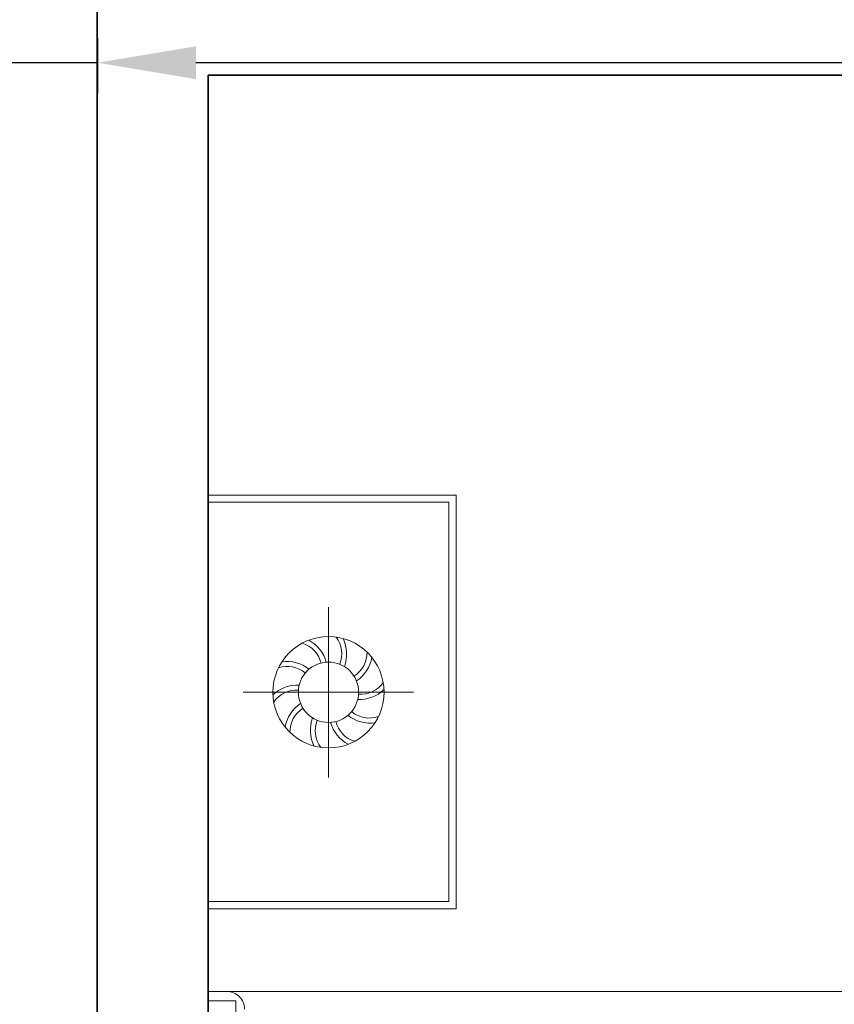
# Model space of a CAD drawing. Units: inches. Extents: x -638 to 186, y -762 to 59.
# Tile 17 of 31: x -168 to -135, y -243 to -203. Entities that reach past the tile are written whole.
import ezdxf

# ---------------------------------------------------------------- set-up
doc = ezdxf.new("R2010")
doc.units = ezdxf.units.IN
for name, color, linetype, lineweight in [('A-ANNO-DIMS', 2, 'Continuous', 18), ('furn', 8, 'Continuous', 13), ('wall', 7, 'Continuous', 35)]:
    doc.layers.add(name, color=color, linetype=linetype, lineweight=lineweight)
doc.styles.get("Standard").update_dxf_attribs({"font": 'arial.ttf'})
doc.dimstyles.new('ISO-25', dxfattribs={"dimtxt": 4, "dimasz": 4, "dimexe": 1.25, "dimexo": 0.625, "dimtad": 0, "dimlunit": 4, "dimtxsty": 'Standard', "dimcen": 2.5, "dimclrt": 256, "dimadec": 0, "dimazin": 0, "dimtfac": 1, "dimtmove": 0, "dimatfit": 3, "dimfxl": 1, "dimfxlon": 1, "dimarcsym": 0})

# ---------------------------------------------------------------- blocks, each defined once
blk = doc.blocks.new('BED-DOUBLE-WITH-NIGHTSTANDS')
for p, q in [((0, 59.951), (78.699, 59.951)), ((58.161, 59.951), (58.161, 58.826)), ((58.548, 11.244), (58.548, 59.951)), ((61.904, 59.951), (61.904, 49.874)), ((62.191, 59.951), (62.191, 50.162)), ((78.411, 50.162), (78.411, 59.951)), ((78.699, 49.874), (78.699, 59.951)), ((58.161, 58.826), (20.398, 58.826)), ((70.694, 51.596), (70.694, 58.516)), ((74.154, 55.056), (67.234, 55.056)), ((62.191, 50.162), (78.411, 50.162)), ((61.904, 49.874), (78.699, 49.874))]:
    blk.add_line(p, q)
for radius in [2.26, 1.225]:
    blk.add_circle((70.694, 55.056), radius)
for centre, radius, start, end in [((57.828, 59.188), 0.72, 270, 0), ((69.67, 56.366), 1.108, 355.462, 55.6998), ((69.537, 56.308), 1.452, 357.5103, 43.83), ((69.022, 55.389), 1.452, 33.5103, 79.83), ((70.636, 56.718), 1.108, 319.462, 19.6998), ((70.494, 56.749), 1.452, 321.5103, 7.83), ((69.096, 55.514), 1.108, 31.462, 91.6998), ((71.623, 56.435), 1.108, 283.462, 343.6998), ((69.132, 54.487), 1.108, 67.462, 127.6998), ((69.146, 54.343), 1.452, 69.5103, 115.83), ((71.527, 56.544), 1.452, 285.5103, 331.83), ((69.861, 53.569), 1.452, 105.5103, 151.83), ((69.765, 53.678), 1.108, 103.462, 163.6998), ((72.242, 55.77), 1.452, 249.5103, 295.83), ((72.256, 55.625), 1.108, 247.462, 307.6998), ((70.894, 53.363), 1.452, 141.5103, 187.83), ((70.753, 53.395), 1.108, 139.462, 199.6998), ((72.292, 54.599), 1.108, 211.462, 271.6998), ((71.851, 53.804), 1.452, 177.5103, 223.83), ((71.718, 53.747), 1.108, 175.462, 235.6998), ((72.366, 54.723), 1.452, 213.5103, 259.83)]:
    blk.add_arc(centre, radius, start, end)
blk = doc.blocks.new('*D23')
at = {"layer": 'A-ANNO-DIMS', "color": 0, "lineweight": -2, "transparency": 16777216}
for p, q in [((-165.015, -204.032), (-165.015, -206.282)), ((-127.219, -204.032), (-127.219, -206.282)), ((-165.015, -205.032), (-169.015, -205.032)), ((-131.219, -205.032), (-161.015, -205.032))]:
    blk.add_line(p, q, dxfattribs=at)
at = {"layer": 'A-ANNO-DIMS', "color": 0, "lineweight": 30, "transparency": 16777216}
for points in [[(-161.015, -204.365), (-161.015, -205.699), (-165.015, -205.032)], [(-131.219, -204.365), (-131.219, -205.699), (-127.219, -205.032)]]:
    blk.add_solid(points, dxfattribs=at)
at = {"layer": 'Defpoints', "color": 0, "lineweight": 30, "transparency": 16777216}
for p in [(-165.015, -199.363), (-127.219, -199.363), (-165.015, -205.032)]:
    blk.add_point(p, dxfattribs=at)
at = {"layer": 'A-ANNO-DIMS', "transparency": 16777216, "insert": (-201.224, -205.032), "char_height": 4, "attachment_point": 5}
blk.add_mtext('SWING DOOR 3\'-2" TYP.', dxfattribs=at)
blk = doc.blocks.new('*D37')
at = {"layer": 'A-ANNO-DIMS', "color": 0, "lineweight": -2, "transparency": 16777216}
for p, q in [((182.663, -232.533), (184.913, -232.533)), ((183.663, -236.533), (183.663, -250.511)), ((183.663, -276.533), (183.663, -262.555)), ((182.663, -280.533), (184.913, -280.533))]:
    blk.add_line(p, q, dxfattribs=at)
at = {"layer": 'A-ANNO-DIMS', "color": 0, "lineweight": 30, "transparency": 16777216}
for points in [[(182.997, -236.533), (184.33, -236.533), (183.663, -232.533)], [(182.997, -276.533), (184.33, -276.533), (183.663, -280.533)]]:
    blk.add_solid(points, dxfattribs=at)
at = {"layer": 'Defpoints', "color": 0, "lineweight": 30, "transparency": 16777216}
for p in [(-404.526, -232.533), (-404.526, -280.533), (183.663, -280.533)]:
    blk.add_point(p, dxfattribs=at)
at = {"layer": 'A-ANNO-DIMS', "transparency": 16777216, "insert": (183.663, -256.533), "char_height": 4, "attachment_point": 5, "rotation": 90}
blk.add_mtext('4\'-0"', dxfattribs=at)
blk = doc.blocks.new('*D56')
at = {"layer": 'A-ANNO-DIMS', "color": 0, "lineweight": -2, "transparency": 16777216}
for p, q in [((-165.026, 52.017), (-165.026, 54.267)), ((-100.526, 52.017), (-100.526, 54.267)), ((-161.026, 53.017), (-143.378, 53.017)), ((-104.526, 53.017), (-122.174, 53.017))]:
    blk.add_line(p, q, dxfattribs=at)
at = {"layer": 'A-ANNO-DIMS', "color": 0, "lineweight": 30, "transparency": 16777216}
for points in [[(-161.026, 53.684), (-161.026, 52.35), (-165.026, 53.017)], [(-104.526, 53.684), (-104.526, 52.35), (-100.526, 53.017)]]:
    blk.add_solid(points, dxfattribs=at)
at = {"layer": 'Defpoints', "color": 0, "lineweight": 30, "transparency": 16777216}
for p in [(-100.526, 53.017), (-165.026, -408.033), (-100.526, -408.033)]:
    blk.add_point(p, dxfattribs=at)
at = {"layer": 'A-ANNO-DIMS', "transparency": 16777216, "insert": (-132.776, 53.017), "char_height": 4, "attachment_point": 5}
blk.add_mtext('5\'-4 1/2"', dxfattribs=at)

msp = doc.modelspace()

# ---------------------------------------------------------------- linework, layer by layer
at = {"layer": 'wall'}
for p, q in [((-165.026, -197.592), (-165.026, -354.033)), ((-160.526, -205.533), (1.474, -205.533)), ((-160.526, -205.533), (-160.526, -349.533))]:
    msp.add_line(p, q, dxfattribs=at)

# ---------------------------------------------------------------- block references
at = {"layer": 'furn', "rotation": 90.00000000000006}
msp.add_blockref('BED-DOUBLE-WITH-NIGHTSTANDS', (-100.575, -301.287), dxfattribs=at)

# ---------------------------------------------------------------- dimensions: what is measured, and where the dimension line sits
at = {"layer": 'A-ANNO-DIMS'}
dim = msp.add_linear_dim(base=(-100.526, 53.017), p1=(-165.026, -408.033), p2=(-100.526, -408.033), dimstyle='ISO-25', override={"dimdec": 1, "dimlfac": 1, "dimrnd": 0, "dimzin": 1, "dimdsep": 46, "dimlunit": 4, "dimfrac": 2}, dxfattribs=at)
dim.commit()
dim.dimension.update_dxf_attribs({"geometry": '*D56', "text_midpoint": (-132.776, 53.017)})
dim = msp.add_linear_dim(base=(-165.015, -205.032), p1=(-127.219, -199.363), p2=(-165.015, -199.363), angle=180, text='SWING DOOR <> TYP.', dimstyle='ISO-25', override={"dimdec": 1, "dimlfac": 1, "dimrnd": 0, "dimzin": 1, "dimdsep": 46, "dimlunit": 4, "dimfrac": 2}, dxfattribs=at)
dim.commit()
dim.dimension.update_dxf_attribs({"geometry": '*D23', "text_midpoint": (-201.224, -205.032)})
dim = msp.add_linear_dim(base=(183.663, -280.533), p1=(-404.526, -232.533), p2=(-404.526, -280.533), angle=90, dimstyle='ISO-25', override={"dimdec": 1, "dimlfac": 1, "dimrnd": 0, "dimzin": 1, "dimdsep": 46, "dimlunit": 4, "dimfrac": 2}, dxfattribs=at)
dim.commit()
dim.dimension.update_dxf_attribs({"geometry": '*D37', "text_midpoint": (183.663, -256.533)})

doc.saveas('drawing.dxf')
